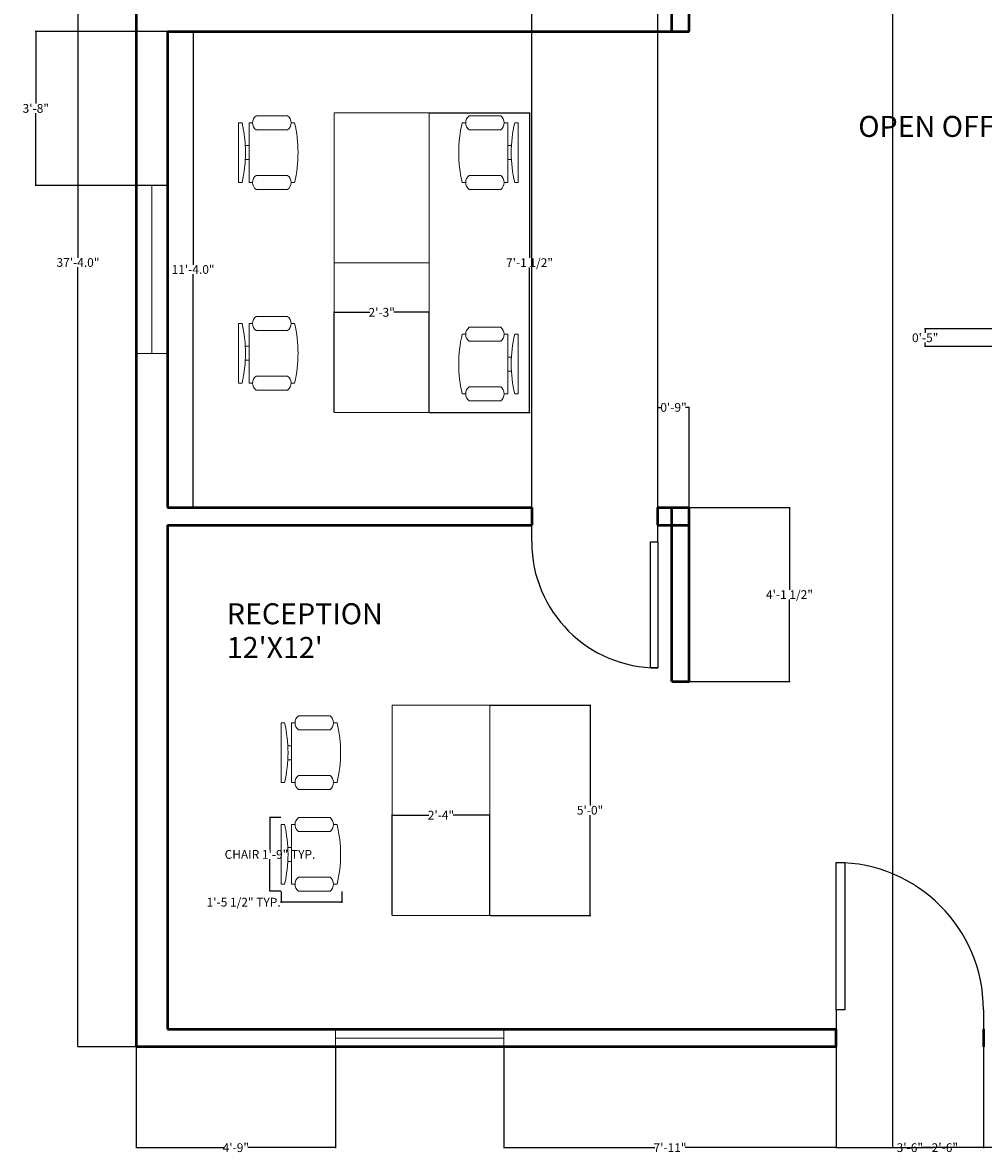
# Model space of a CAD drawing. Units: inches. Extents: x 9441 to 10027, y 18319 to 18830.
# Tile 1 of 4: x 9441 to 9716, y 18319 to 18642. Entities that reach past the tile are written whole.
import ezdxf

# ---------------------------------------------------------------- set-up
doc = ezdxf.new("R2010")
doc.units = ezdxf.units.IN
doc.header["$MEASUREMENT"] = 0
for name, color, linetype, lineweight in [('A-ANNO-DIMS', 2, 'Continuous', 18), ('A-AREA-IDEN', 7, 'Continuous', 25), ('A-DOOR', 3, 'Continuous', 25), ('A-GLAZ', 4, 'Continuous', 18), ('A-WALL', 7, 'Continuous', 50), ('furniture', 8, 'Continuous', 18)]:
    doc.layers.add(name, color=color, linetype=linetype, lineweight=lineweight)
doc.styles.get("Standard").update_dxf_attribs({"font": 'arial.ttf'})
doc.dimstyles.get("Standard").update_dxf_attribs({"dimtxt": 2.5, "dimasz": 0.18, "dimexe": 0.18, "dimexo": 0.0625, "dimgap": 0.09, "dimtad": 0, "dimtih": 1, "dimtoh": 1, "dimdec": 1, "dimzin": 0, "dimdsep": 46, "dimlunit": 3, "dimtxsty": 'Standard', "dimcen": 0.09, "dimadec": 0, "dimazin": 0, "dimtfac": 1, "dimtdec": 1, "dimtofl": 0, "dimtmove": 0, "dimatfit": 3, "dimfxl": 1, "dimtolj": 1, "dimtzin": 0, "dimarcsym": 0})

# ---------------------------------------------------------------- blocks, each defined once
blk = doc.blocks.new('*U2')
for p, q in [((0, 0), (0, -100)), ((750, 0), (750, -100))]:
    blk.add_line(p, q)
blk.add_lwpolyline([(0, 0), (0, 750), (43.75, 750), (43.75, 0)], close=True)
blk.add_arc((0, 0), 750, 0, 90)
blk = doc.blocks.new('*U4')
for p, q in [((0, 100), (0, 0)), ((900, 100), (900, 0)), ((0, 50), (900, 50))]:
    blk.add_line(p, q)
blk = doc.blocks.new('Chair - Desk')
for p, q in [((-8.5, 0), (-8.5, -1)), ((-8.5, 0), (8.5, 0)), ((8.5, 0), (8.5, -1)), ((-8.5, -3), (-8.5, -4)), ((-8.5, -3), (8.5, -3)), ((-2, -3), (-2, -1.9355)), ((2, -1.9576), (2, -3)), ((8.5, -3), (8.5, -4)), ((-10.5, -5), (-10.5, -14)), ((-6.5, -14), (-6.5, -5)), ((6.5, -5), (6.5, -14)), ((10.5, -14), (10.5, -5)), ((-8.5, -15), (-8.5, -16)), ((8.5, -15), (8.5, -16))]:
    blk.add_line(p, q)
for centre, radius, start, end in [((0, 34.625), 36.625, 256.5803, 283.4197), ((-8.5, -6.5), 2.5, 36.8699, 143.1301), ((8.5, -6.5), 2.5, 36.8699, 143.1301), ((-8.5, -12.5), 2.5, 216.8699, 323.1301), ((0, 19.625), 36.625, 256.5803, 283.4197), ((8.5, -12.5), 2.5, 216.8699, 323.1301)]:
    blk.add_arc(centre, radius, start, end)
blk = doc.blocks.new('*D13')
at = {"layer": 'A-ANNO-DIMS', "color": 0, "lineweight": -2, "transparency": 16777216}
for p, q in [((9482.95, 18639.93), (9490.37, 18639.93)), ((9490.19, 18639.75), (9490.19, 18573.29)), ((9490.19, 18504.11), (9490.19, 18570.56)), ((9482.95, 18503.93), (9490.37, 18503.93))]:
    blk.add_line(p, q, dxfattribs=at)
at = {"layer": 'A-ANNO-DIMS', "color": 0, "transparency": 16777216}
for points in [[(9490.16, 18639.75), (9490.22, 18639.75), (9490.19, 18639.93)], [(9490.16, 18504.11), (9490.22, 18504.11), (9490.19, 18503.93)]]:
    blk.add_solid(points, dxfattribs=at)
at = {"layer": 'Defpoints', "color": 0, "transparency": 16777216}
for p in [(9482.89, 18639.93), (9482.89, 18503.93), (9490.19, 18503.93)]:
    blk.add_point(p, dxfattribs=at)
at = {"layer": 'A-ANNO-DIMS', "color": 0, "transparency": 16777216, "insert": (9490.19, 18571.93), "char_height": 2.5, "attachment_point": 5}
blk.add_mtext('\\A1;11\'-4.0"', dxfattribs=at)
blk = doc.blocks.new('*D15')
at = {"layer": 'A-ANNO-DIMS', "color": 0, "lineweight": -2, "transparency": 16777216}
for p, q in [((9473.83, 18797.93), (9457.13, 18797.93)), ((9457.31, 18797.75), (9457.31, 18575.29)), ((9457.31, 18350.11), (9457.31, 18572.56)), ((9473.83, 18349.93), (9457.13, 18349.93))]:
    blk.add_line(p, q, dxfattribs=at)
at = {"layer": 'A-ANNO-DIMS', "color": 0, "transparency": 16777216}
for points in [[(9457.28, 18797.75), (9457.34, 18797.75), (9457.31, 18797.93)], [(9457.28, 18350.11), (9457.34, 18350.11), (9457.31, 18349.93)]]:
    blk.add_solid(points, dxfattribs=at)
at = {"layer": 'Defpoints', "color": 0, "transparency": 16777216}
for p in [(9473.89, 18797.93), (9457.31, 18349.93), (9473.89, 18349.93)]:
    blk.add_point(p, dxfattribs=at)
at = {"layer": 'A-ANNO-DIMS', "color": 0, "transparency": 16777216, "insert": (9457.31, 18573.93), "char_height": 2.5, "attachment_point": 5}
blk.add_mtext('\\A1;37\'-4.0"', dxfattribs=at)
blk = doc.blocks.new('WIN-FRAME-48x9')
for p, q in [((48, 9), (0, 9)), ((0, 9), (0, 0)), ((48, 0), (48, 9))]:
    blk.add_line(p, q)
blk = doc.blocks.new('*D21')
at = {"layer": 'A-ANNO-DIMS', "color": 0, "lineweight": -2, "transparency": 16777216}
for p, q in [((9515.24, 18415.38), (9511.97, 18415.38)), ((9512.15, 18415.2), (9512.15, 18406.26)), ((9512.15, 18394.56), (9512.15, 18403.5)), ((9515.24, 18394.38), (9511.97, 18394.38))]:
    blk.add_line(p, q, dxfattribs=at)
at = {"layer": 'A-ANNO-DIMS', "color": 0, "transparency": 16777216}
for points in [[(9512.12, 18415.2), (9512.18, 18415.2), (9512.15, 18415.38)], [(9512.12, 18394.56), (9512.18, 18394.56), (9512.15, 18394.38)]]:
    blk.add_solid(points, dxfattribs=at)
at = {"layer": 'Defpoints', "color": 0, "transparency": 16777216}
for p in [(9512.15, 18415.38), (9515.3, 18415.38), (9515.3, 18394.38)]:
    blk.add_point(p, dxfattribs=at)
at = {"layer": 'A-ANNO-DIMS', "color": 0, "transparency": 16777216, "insert": (9512.15, 18404.88), "char_height": 2.5, "attachment_point": 5}
blk.add_mtext('\\A1;CHAIR 1\'-9" TYP.', dxfattribs=at)
blk = doc.blocks.new('*D22')
at = {"layer": 'A-ANNO-DIMS', "color": 0, "lineweight": -2, "transparency": 16777216}
for p, q in [((9515.3, 18394.32), (9515.3, 18391.05)), ((9532.64, 18394.32), (9532.64, 18391.05)), ((9515.3, 18391.23), (9515.12, 18391.23)), ((9532.46, 18391.23), (9515.48, 18391.23))]:
    blk.add_line(p, q, dxfattribs=at)
at = {"layer": 'A-ANNO-DIMS', "color": 0, "transparency": 16777216}
for points in [[(9515.48, 18391.26), (9515.48, 18391.2), (9515.3, 18391.23)], [(9532.46, 18391.26), (9532.46, 18391.2), (9532.64, 18391.23)]]:
    blk.add_solid(points, dxfattribs=at)
at = {"layer": 'Defpoints', "color": 0, "transparency": 16777216}
for p in [(9515.3, 18394.38), (9532.64, 18394.38), (9515.3, 18391.23)]:
    blk.add_point(p, dxfattribs=at)
at = {"layer": 'A-ANNO-DIMS', "color": 0, "transparency": 16777216, "insert": (9504.62, 18391.23), "char_height": 2.5, "attachment_point": 5}
blk.add_mtext('\\A1;1\'-5 1/2" TYP.', dxfattribs=at)
blk = doc.blocks.new('*D38')
at = {"layer": 'A-ANNO-DIMS', "color": 0, "lineweight": -2, "transparency": 16777216}
for p, q in [((9473.89, 18349.86), (9473.89, 18320.95)), ((9530.89, 18349.86), (9530.89, 18320.95)), ((9474.07, 18321.13), (9498.93, 18321.13)), ((9530.71, 18321.13), (9505.85, 18321.13))]:
    blk.add_line(p, q, dxfattribs=at)
at = {"layer": 'A-ANNO-DIMS', "color": 0, "transparency": 16777216}
for points in [[(9474.07, 18321.16), (9474.07, 18321.1), (9473.89, 18321.13)], [(9530.71, 18321.16), (9530.71, 18321.1), (9530.89, 18321.13)]]:
    blk.add_solid(points, dxfattribs=at)
at = {"layer": 'Defpoints', "color": 0, "transparency": 16777216}
for p in [(9473.89, 18349.93), (9530.89, 18349.93), (9530.89, 18321.13)]:
    blk.add_point(p, dxfattribs=at)
at = {"layer": 'A-ANNO-DIMS', "color": 0, "transparency": 16777216, "insert": (9502.39, 18321.13), "char_height": 2.5, "attachment_point": 5}
blk.add_mtext('\\A1;4\'-9"', dxfattribs=at)
blk = doc.blocks.new('*D39')
at = {"layer": 'A-ANNO-DIMS', "color": 0, "lineweight": -2, "transparency": 16777216}
for p, q in [((9578.89, 18349.86), (9578.89, 18320.95)), ((9673.89, 18349.86), (9673.89, 18320.95)), ((9579.07, 18321.13), (9622.02, 18321.13)), ((9673.71, 18321.13), (9630.76, 18321.13))]:
    blk.add_line(p, q, dxfattribs=at)
at = {"layer": 'A-ANNO-DIMS', "color": 0, "transparency": 16777216}
for points in [[(9579.07, 18321.16), (9579.07, 18321.1), (9578.89, 18321.13)], [(9673.71, 18321.16), (9673.71, 18321.1), (9673.89, 18321.13)]]:
    blk.add_solid(points, dxfattribs=at)
at = {"layer": 'Defpoints', "color": 0, "transparency": 16777216}
for p in [(9578.89, 18349.93), (9673.89, 18349.93), (9673.89, 18321.13)]:
    blk.add_point(p, dxfattribs=at)
at = {"layer": 'A-ANNO-DIMS', "color": 0, "transparency": 16777216, "insert": (9626.39, 18321.13), "char_height": 2.5, "attachment_point": 5}
blk.add_mtext('\\A1;7\'-11"', dxfattribs=at)
blk = doc.blocks.new('*D40')
at = {"layer": 'A-ANNO-DIMS', "color": 0, "lineweight": -2, "transparency": 16777216}
for p, q in [((9673.89, 18349.86), (9673.89, 18320.95)), ((9715.89, 18349.86), (9715.89, 18320.95)), ((9674.07, 18321.13), (9691.48, 18321.13)), ((9715.71, 18321.13), (9698.3, 18321.13))]:
    blk.add_line(p, q, dxfattribs=at)
at = {"layer": 'A-ANNO-DIMS', "color": 0, "transparency": 16777216}
for points in [[(9674.07, 18321.16), (9674.07, 18321.1), (9673.89, 18321.13)], [(9715.71, 18321.16), (9715.71, 18321.1), (9715.89, 18321.13)]]:
    blk.add_solid(points, dxfattribs=at)
at = {"layer": 'Defpoints', "color": 0, "transparency": 16777216}
for p in [(9673.89, 18349.93), (9715.89, 18349.93), (9715.89, 18321.13)]:
    blk.add_point(p, dxfattribs=at)
at = {"layer": 'A-ANNO-DIMS', "color": 0, "transparency": 16777216, "insert": (9694.89, 18321.13), "char_height": 2.5, "attachment_point": 5}
blk.add_mtext('\\A1;3\'-6"', dxfattribs=at)
blk = doc.blocks.new('*D45')
at = {"layer": 'A-ANNO-DIMS', "color": 0, "lineweight": -2, "transparency": 16777216}
for p, q in [((9482.83, 18639.93), (9445.09, 18639.93)), ((9445.27, 18639.75), (9445.27, 18619.29)), ((9445.27, 18596.11), (9445.27, 18616.56)), ((9482.83, 18595.93), (9445.09, 18595.93))]:
    blk.add_line(p, q, dxfattribs=at)
at = {"layer": 'A-ANNO-DIMS', "color": 0, "transparency": 16777216}
for points in [[(9445.24, 18639.75), (9445.3, 18639.75), (9445.27, 18639.93)], [(9445.24, 18596.11), (9445.3, 18596.11), (9445.27, 18595.93)]]:
    blk.add_solid(points, dxfattribs=at)
at = {"layer": 'Defpoints', "color": 0, "transparency": 16777216}
for p in [(9445.27, 18639.93), (9482.89, 18639.93), (9482.89, 18595.93)]:
    blk.add_point(p, dxfattribs=at)
at = {"layer": 'A-ANNO-DIMS', "color": 0, "transparency": 16777216, "insert": (9445.27, 18617.93), "char_height": 2.5, "attachment_point": 5}
blk.add_mtext('\\A1;3\'-8"', dxfattribs=at)
blk = doc.blocks.new('*D47')
at = {"layer": 'A-ANNO-DIMS', "color": 0, "lineweight": -2, "transparency": 16777216}
for p, q in [((9689.89, 18687.86), (9689.89, 18320.95)), ((9719.89, 18687.86), (9719.89, 18320.95)), ((9690.07, 18321.13), (9701.46, 18321.13)), ((9719.71, 18321.13), (9708.32, 18321.13))]:
    blk.add_line(p, q, dxfattribs=at)
at = {"layer": 'A-ANNO-DIMS', "color": 0, "transparency": 16777216}
for points in [[(9690.07, 18321.16), (9690.07, 18321.1), (9689.89, 18321.13)], [(9719.71, 18321.16), (9719.71, 18321.1), (9719.89, 18321.13)]]:
    blk.add_solid(points, dxfattribs=at)
at = {"layer": 'Defpoints', "color": 0, "transparency": 16777216}
for p in [(9689.89, 18687.93), (9719.89, 18687.93), (9719.89, 18321.13)]:
    blk.add_point(p, dxfattribs=at)
at = {"layer": 'A-ANNO-DIMS', "color": 0, "transparency": 16777216, "insert": (9704.89, 18321.13), "char_height": 2.5, "attachment_point": 5}
blk.add_mtext('\\A1;2\'-6"', dxfattribs=at)
blk = doc.blocks.new('*D54')
at = {"layer": 'A-ANNO-DIMS', "color": 0, "lineweight": -2, "transparency": 16777216}
for p, q in [((9631.952882, 18503.92582), (9660.695382, 18503.92582)), ((9660.515382, 18503.74582), (9660.515382, 18480.450916)), ((9660.515382, 18454.390746), (9660.515382, 18477.68565)), ((9631.952882, 18454.210746), (9660.695382, 18454.210746))]:
    blk.add_line(p, q, dxfattribs=at)
at = {"layer": 'A-ANNO-DIMS', "color": 0, "transparency": 16777216}
for points in [[(9660.485382, 18503.74582), (9660.545382, 18503.74582), (9660.515382, 18503.92582)], [(9660.485382, 18454.390746), (9660.545382, 18454.390746), (9660.515382, 18454.210746)]]:
    blk.add_solid(points, dxfattribs=at)
at = {"layer": 'Defpoints', "color": 0, "transparency": 16777216}
for p in [(9631.890382, 18503.92582), (9631.890382, 18454.210746), (9660.515382, 18454.210746)]:
    blk.add_point(p, dxfattribs=at)
at = {"layer": 'A-ANNO-DIMS', "color": 0, "transparency": 16777216, "insert": (9660.515382, 18479.068283), "char_height": 2.5, "attachment_point": 5}
blk.add_mtext('\\A1;4\'-1 1/2"', dxfattribs=at)
blk = doc.blocks.new('*D55')
at = {"layer": 'A-ANNO-DIMS', "color": 0, "lineweight": -2, "transparency": 16777216}
for p, q in [((9586.89, 18503.99), (9586.89, 18826.73)), ((9587.07, 18826.55), (9601.48, 18826.55)), ((9622.71, 18826.55), (9608.3, 18826.55)), ((9622.89, 18503.99), (9622.89, 18826.73))]:
    blk.add_line(p, q, dxfattribs=at)
at = {"layer": 'A-ANNO-DIMS', "color": 0, "transparency": 16777216}
for points in [[(9587.07, 18826.58), (9587.07, 18826.52), (9586.89, 18826.55)], [(9622.71, 18826.58), (9622.71, 18826.52), (9622.89, 18826.55)]]:
    blk.add_solid(points, dxfattribs=at)
at = {"layer": 'Defpoints', "color": 0, "transparency": 16777216}
for p in [(9622.89, 18826.55), (9586.89, 18503.93), (9622.89, 18503.93)]:
    blk.add_point(p, dxfattribs=at)
at = {"layer": 'A-ANNO-DIMS', "color": 0, "transparency": 16777216, "insert": (9604.89, 18826.55), "char_height": 2.5, "attachment_point": 5}
blk.add_mtext('\\A1;3\'-0"', dxfattribs=at)
blk = doc.blocks.new('*D57')
at = {"layer": 'A-ANNO-DIMS', "color": 0, "lineweight": -2, "transparency": 16777216}
for p, q in [((9727.83, 18554.93), (9699.09, 18554.93)), ((9699.27, 18554.75), (9699.27, 18553.79)), ((9727.83, 18549.93), (9699.09, 18549.93)), ((9699.27, 18550.11), (9699.27, 18551.06))]:
    blk.add_line(p, q, dxfattribs=at)
at = {"layer": 'A-ANNO-DIMS', "color": 0, "transparency": 16777216}
for points in [[(9699.24, 18554.75), (9699.3, 18554.75), (9699.27, 18554.93)], [(9699.24, 18550.11), (9699.3, 18550.11), (9699.27, 18549.93)]]:
    blk.add_solid(points, dxfattribs=at)
at = {"layer": 'Defpoints', "color": 0, "transparency": 16777216}
for p in [(9699.27, 18554.93), (9727.89, 18554.93), (9727.89, 18549.93)]:
    blk.add_point(p, dxfattribs=at)
at = {"layer": 'A-ANNO-DIMS', "color": 0, "transparency": 16777216, "insert": (9699.27, 18552.43), "char_height": 2.5, "attachment_point": 5}
blk.add_mtext('\\A1;0\'-5"', dxfattribs=at)
blk = doc.blocks.new('*D58')
at = {"layer": 'A-ANNO-DIMS', "color": 0, "lineweight": -2, "transparency": 16777216}
for p, q in [((9547.03, 18387.53), (9547.03, 18416.27)), ((9547.21, 18416.09), (9557.55, 18416.09)), ((9574.76, 18416.09), (9564.42, 18416.09)), ((9574.94, 18387.53), (9574.94, 18416.27))]:
    blk.add_line(p, q, dxfattribs=at)
at = {"layer": 'A-ANNO-DIMS', "color": 0, "transparency": 16777216}
for points in [[(9547.21, 18416.12), (9547.21, 18416.06), (9547.03, 18416.09)], [(9574.76, 18416.12), (9574.76, 18416.06), (9574.94, 18416.09)]]:
    blk.add_solid(points, dxfattribs=at)
at = {"layer": 'Defpoints', "color": 0, "transparency": 16777216}
for p in [(9574.94, 18416.09), (9547.03, 18387.47), (9574.94, 18387.47)]:
    blk.add_point(p, dxfattribs=at)
at = {"layer": 'A-ANNO-DIMS', "color": 0, "transparency": 16777216, "insert": (9560.98, 18416.09), "char_height": 2.5, "attachment_point": 5}
blk.add_mtext('\\A1;2\'-4"', dxfattribs=at)
blk = doc.blocks.new('*D59')
at = {"layer": 'A-ANNO-DIMS', "color": 0, "lineweight": -2, "transparency": 16777216}
for p, q in [((9575, 18447.51), (9603.74, 18447.51)), ((9603.56, 18447.33), (9603.56, 18418.85)), ((9603.56, 18387.65), (9603.56, 18416.12)), ((9575, 18387.47), (9603.74, 18387.47))]:
    blk.add_line(p, q, dxfattribs=at)
at = {"layer": 'A-ANNO-DIMS', "color": 0, "transparency": 16777216}
for points in [[(9603.53, 18447.33), (9603.59, 18447.33), (9603.56, 18447.51)], [(9603.53, 18387.65), (9603.59, 18387.65), (9603.56, 18387.47)]]:
    blk.add_solid(points, dxfattribs=at)
at = {"layer": 'Defpoints', "color": 0, "transparency": 16777216}
for p in [(9574.94, 18447.51), (9574.94, 18387.47), (9603.56, 18387.47)]:
    blk.add_point(p, dxfattribs=at)
at = {"layer": 'A-ANNO-DIMS', "color": 0, "transparency": 16777216, "insert": (9603.56, 18417.49), "char_height": 2.5, "attachment_point": 5}
blk.add_mtext('\\A1;5\'-0"', dxfattribs=at)
blk = doc.blocks.new('*D60')
at = {"layer": 'A-ANNO-DIMS', "color": 0, "lineweight": -2, "transparency": 16777216}
for p, q in [((9530.45, 18531.13), (9530.45, 18559.87)), ((9530.63, 18559.69), (9540.62, 18559.69)), ((9557.47, 18559.69), (9547.48, 18559.69)), ((9557.65, 18531.13), (9557.65, 18559.87))]:
    blk.add_line(p, q, dxfattribs=at)
at = {"layer": 'A-ANNO-DIMS', "color": 0, "transparency": 16777216}
for points in [[(9530.63, 18559.72), (9530.63, 18559.66), (9530.45, 18559.69)], [(9557.47, 18559.72), (9557.47, 18559.66), (9557.65, 18559.69)]]:
    blk.add_solid(points, dxfattribs=at)
at = {"layer": 'Defpoints', "color": 0, "transparency": 16777216}
for p in [(9557.65, 18559.69), (9530.45, 18531.06), (9557.65, 18531.06)]:
    blk.add_point(p, dxfattribs=at)
at = {"layer": 'A-ANNO-DIMS', "color": 0, "transparency": 16777216, "insert": (9544.05, 18559.69), "char_height": 2.5, "attachment_point": 5}
blk.add_mtext('\\A1;2\'-3"', dxfattribs=at)
blk = doc.blocks.new('*D61')
at = {"layer": 'A-ANNO-DIMS', "color": 0, "lineweight": -2, "transparency": 16777216}
for p, q in [((9557.71, 18616.67), (9586.45, 18616.67)), ((9586.27, 18616.49), (9586.27, 18575.25)), ((9586.27, 18531.24), (9586.27, 18572.49)), ((9557.71, 18531.06), (9586.45, 18531.06))]:
    blk.add_line(p, q, dxfattribs=at)
at = {"layer": 'A-ANNO-DIMS', "color": 0, "transparency": 16777216}
for points in [[(9586.24, 18616.49), (9586.3, 18616.49), (9586.27, 18616.67)], [(9586.24, 18531.24), (9586.3, 18531.24), (9586.27, 18531.06)]]:
    blk.add_solid(points, dxfattribs=at)
at = {"layer": 'Defpoints', "color": 0, "transparency": 16777216}
for p in [(9557.65, 18616.67), (9557.65, 18531.06), (9586.27, 18531.06)]:
    blk.add_point(p, dxfattribs=at)
at = {"layer": 'A-ANNO-DIMS', "color": 0, "transparency": 16777216, "insert": (9586.27, 18573.87), "char_height": 2.5, "attachment_point": 5}
blk.add_mtext('\\A1;7\'-1 1/2"', dxfattribs=at)
blk = doc.blocks.new('*D71')
at = {"layer": 'A-ANNO-DIMS', "color": 0, "lineweight": -2, "transparency": 16777216}
for p, q in [((9622.89, 18503.99), (9622.89, 18532.73)), ((9623.07, 18532.55), (9623.98, 18532.55)), ((9631.71, 18532.55), (9630.8, 18532.55)), ((9631.89, 18503.99), (9631.89, 18532.73))]:
    blk.add_line(p, q, dxfattribs=at)
at = {"layer": 'A-ANNO-DIMS', "color": 0, "transparency": 16777216}
for points in [[(9623.07, 18532.58), (9623.07, 18532.52), (9622.89, 18532.55)], [(9631.71, 18532.58), (9631.71, 18532.52), (9631.89, 18532.55)]]:
    blk.add_solid(points, dxfattribs=at)
at = {"layer": 'Defpoints', "color": 0, "transparency": 16777216}
for p in [(9631.89, 18532.55), (9622.89, 18503.93), (9631.89, 18503.93)]:
    blk.add_point(p, dxfattribs=at)
at = {"layer": 'A-ANNO-DIMS', "color": 0, "transparency": 16777216, "insert": (9627.39, 18532.55), "char_height": 2.5, "attachment_point": 5}
blk.add_mtext('\\A1;0\'-9"', dxfattribs=at)

msp = doc.modelspace()

# ---------------------------------------------------------------- linework, layer by layer
at = {"layer": 'A-GLAZ'}
for p, q in [((9530.89, 18354.93), (9530.89, 18349.93)), ((9578.89, 18349.93), (9578.89, 18354.93)), ((9530.89, 18349.93), (9578.89, 18349.93))]:
    msp.add_line(p, q, dxfattribs=at)
at = {"layer": 'A-WALL'}
for p, q in [((9473.89, 18797.93), (9473.89, 18349.93)), ((9626.89, 18639.93), (9626.89, 18648.93)), ((9631.89, 18639.93), (9631.89, 18648.93)), ((9482.89, 18639.93), (9631.89, 18639.93)), ((9482.89, 18639.93), (9482.89, 18503.93)), ((9482.89, 18503.93), (9586.89, 18503.93)), ((9586.89, 18503.93), (9586.89, 18498.93)), ((9622.89, 18498.93), (9622.89, 18503.93)), ((9622.89, 18503.93), (9631.89, 18503.93)), ((9626.89, 18454.21), (9626.89, 18503.93)), ((9631.89, 18454.21), (9631.89, 18503.93)), ((9482.89, 18498.93), (9586.89, 18498.93)), ((9482.89, 18498.93), (9482.89, 18354.93)), ((9622.89, 18498.93), (9631.89, 18498.93)), ((9626.89, 18454.21), (9631.89, 18454.21)), ((9482.89, 18354.93), (9673.89, 18354.93)), ((9673.89, 18349.93), (9673.89, 18354.93)), ((9715.89, 18354.93), (9715.89, 18349.93)), ((9673.89, 18349.93), (9473.89, 18349.93))]:
    msp.add_line(p, q, dxfattribs=at)
at = {"layer": 'furniture'}
msp.add_line((9557.65, 18573.87), (9530.45, 18573.87), dxfattribs=at)
for points in [[(9530.45, 18616.67), (9557.65, 18616.67), (9557.65, 18531.06), (9530.45, 18531.06)], [(9547.03, 18447.51), (9574.94, 18447.51), (9574.94, 18387.47), (9547.03, 18387.47)]]:
    msp.add_lwpolyline(points, close=True, dxfattribs=at)

# ---------------------------------------------------------------- block references
at = {"layer": 'A-DOOR', "xscale": 0.0480000000000006, "yscale": 0.0480000000000006, "zscale": 0.0480000000000006, "rotation": 180}
msp.add_blockref('*U2', (9622.89, 18494.13), dxfattribs=at)
at = {"layer": 'A-DOOR', "xscale": 0.0560000000000007, "yscale": 0.0560000000000007, "zscale": 0.0560000000000007}
msp.add_blockref('*U2', (9673.89, 18360.53), dxfattribs=at)
at = {"layer": 'A-GLAZ', "rotation": 89.99999999999898}
msp.add_blockref('WIN-FRAME-48x9', (9482.89, 18547.93), dxfattribs=at)
at = {"layer": 'A-GLAZ', "xscale": 0.0533333333333332, "yscale": 0.0533333333333332, "zscale": 0.0533333333333332, "rotation": 270}
msp.add_blockref('*U4', (9475.72, 18595.93), dxfattribs=at)
at = {"layer": 'A-GLAZ', "xscale": 0.0533333333333332, "yscale": 0.0533333333333332, "zscale": 0.0533333333333332}
msp.add_blockref('*U4', (9530.89, 18349.76), dxfattribs=at)
at = {"layer": 'furniture'}
for p, rotation in [((9503.16, 18605.29), 90), ((9583.04, 18605.29), 270), ((9503.16, 18548), 90), ((9583.04, 18544.91), 270), ((9515.3, 18433.93), 90), ((9515.3, 18404.88), 90)]:
    msp.add_blockref('Chair - Desk', p, dxfattribs=dict(at, rotation=rotation))

# ---------------------------------------------------------------- texts
at = {"layer": 'A-AREA-IDEN'}
for s, p in [('OPEN OFFICE AREA', (9680.17, 18609.79)), ('RECEPTION', (9499.81, 18470.6)), ("12'X12'", (9499.81, 18460.96))]:
    msp.add_text(s, height=6, dxfattribs=at).set_placement(p)

# ---------------------------------------------------------------- dimensions: what is measured, and where the dimension line sits
at = {"layer": 'A-ANNO-DIMS'}
for base, p1, p2, picture, middle in [((9622.89, 18826.55), (9586.89, 18503.93), (9622.89, 18503.93), '*D55', (9604.89, 18826.55)), ((9719.89, 18321.13), (9689.89, 18687.93), (9719.89, 18687.93), '*D47', (9704.89, 18321.13)), ((9557.65, 18559.69), (9530.45, 18531.06), (9557.65, 18531.06), '*D60', (9544.05, 18559.69)), ((9631.89, 18532.55), (9622.89, 18503.93), (9631.89, 18503.93), '*D71', (9627.39, 18532.55)), ((9574.94, 18416.09), (9547.03, 18387.47), (9574.94, 18387.47), '*D58', (9560.98, 18416.09)), ((9530.89, 18321.13), (9473.89, 18349.93), (9530.89, 18349.93), '*D38', (9502.39, 18321.13)), ((9673.89, 18321.13), (9578.89, 18349.93), (9673.89, 18349.93), '*D39', (9626.39, 18321.13)), ((9715.89, 18321.13), (9673.89, 18349.93), (9715.89, 18349.93), '*D40', (9694.89, 18321.13))]:
    dim = msp.add_linear_dim(base=base, p1=p1, p2=p2, dimstyle='Standard', override={"dimdec": 1, "dimlfac": 1, "dimrnd": 0, "dimzin": 1, "dimdsep": 46, "dimlunit": 4, "dimfrac": 2}, dxfattribs=at)
    dim.commit()
    dim.dimension.update_dxf_attribs({"geometry": picture, "text_midpoint": middle})
for base, p1, p2, angle, override, picture, middle in [((9457.31, 18349.93), (9473.89, 18797.93), (9473.89, 18349.93), 90, {"dimclrd": 0, "dimclre": 0, "dimclrt": 0}, '*D15', (9457.31, 18573.93)), ((9445.27, 18639.93), (9482.89, 18595.93), (9482.89, 18639.93), 90, {"dimdec": 1, "dimlfac": 1, "dimrnd": 0, "dimzin": 1, "dimdsep": 46, "dimlunit": 4, "dimfrac": 2}, '*D45', (9445.27, 18617.93)), ((9490.19, 18503.93), (9482.89, 18639.93), (9482.89, 18503.93), 90, {"dimclrd": 0, "dimclre": 0, "dimclrt": 0}, '*D13', (9490.19, 18571.93)), ((9586.27, 18531.06), (9557.65, 18616.67), (9557.65, 18531.06), 270, {"dimdec": 1, "dimlfac": 1, "dimrnd": 0, "dimzin": 1, "dimdsep": 46, "dimlunit": 4, "dimfrac": 2}, '*D61', (9586.27, 18573.87)), ((9699.27, 18554.93), (9727.89, 18549.93), (9727.89, 18554.93), 90, {"dimdec": 1, "dimlfac": 1, "dimrnd": 0, "dimzin": 1, "dimdsep": 46, "dimlunit": 4, "dimfrac": 2}, '*D57', (9699.27, 18552.43)), ((9660.52, 18454.21), (9631.89, 18503.93), (9631.89, 18454.21), 270, {"dimdec": 1, "dimlfac": 1, "dimrnd": 0, "dimzin": 1, "dimdsep": 46, "dimlunit": 4, "dimfrac": 2}, '*D54', (9660.52, 18479.07)), ((9603.56, 18387.47), (9574.94, 18447.51), (9574.94, 18387.47), 270, {"dimdec": 1, "dimlfac": 1, "dimrnd": 0, "dimzin": 1, "dimdsep": 46, "dimlunit": 4, "dimfrac": 2}, '*D59', (9603.56, 18417.49))]:
    dim = msp.add_linear_dim(base=base, p1=p1, p2=p2, angle=angle, dimstyle='Standard', override=override, dxfattribs=at)
    dim.commit()
    dim.dimension.update_dxf_attribs({"geometry": picture, "text_midpoint": middle})
for base, p1, p2, angle, text, picture, middle in [((9512.15, 18415.38), (9515.3, 18394.38), (9515.3, 18415.38), 90, 'CHAIR <> TYP.', '*D21', (9512.15, 18404.88)), ((9515.3, 18391.23), (9532.64, 18394.38), (9515.3, 18394.38), 180, '<> TYP.', '*D22', (9504.62, 18391.23))]:
    dim = msp.add_linear_dim(base=base, p1=p1, p2=p2, angle=angle, text=text, dimstyle='Standard', override={"dimdec": 1, "dimlfac": 1, "dimrnd": 0, "dimzin": 1, "dimdsep": 46, "dimlunit": 4, "dimfrac": 2}, dxfattribs=at)
    dim.commit()
    dim.dimension.update_dxf_attribs({"geometry": picture, "text_midpoint": middle})

doc.saveas('drawing.dxf')
